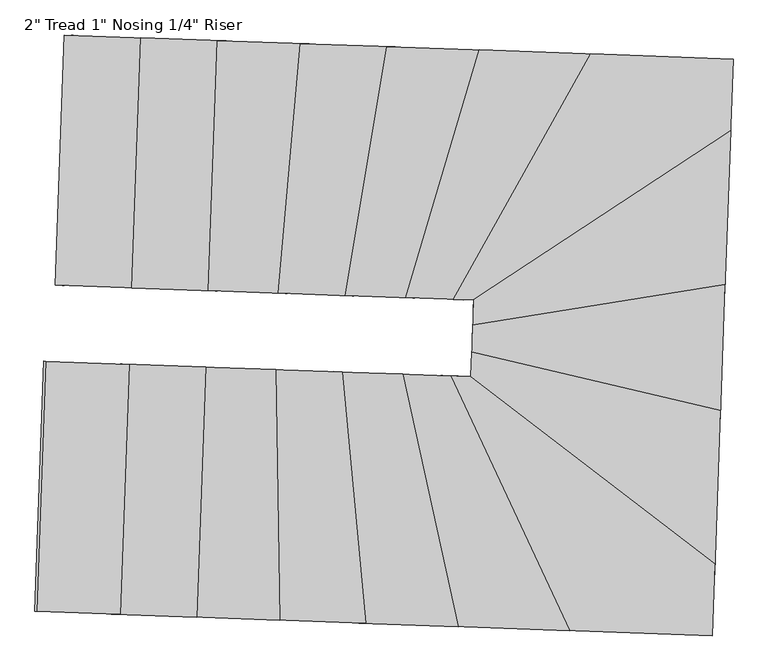
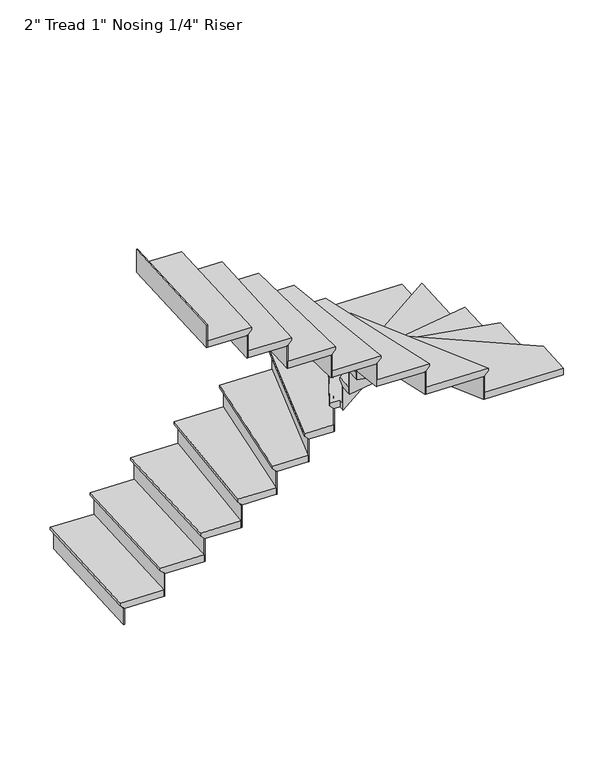
"""IFC4 building model written with IfcOpenShell, lengths in millimetres: stair flight geometry."""

from ifc_helpers import new_model, si_unit, origin, place, context, project, spatial, faceted_brep, source, transform, mapped, element, save


def stair_flight_9054a24f(model_context):
    return source(origin(), model_context, "Body", "Brep", [
        faceted_brep([(-10039.2744432, -1277.1215258, 150.2833333), (-10039.2744432, -1277.1215258, 169.3333333), (-10006.394185, -363.3128759, 169.3333333), (-10006.394185, -363.3128759, 150.2833333), (-10013.8908696, -1278.0348663, 124.8833333), (-9981.0106114, -364.2262164, 124.8833333), (-9734.6715599, -1288.0816118, 169.3333333), (-9701.7913017, -374.272962, 169.3333333), (-9981.0106114, -364.2262164, 118.5333333), (-9701.7913017, -374.272962, 118.5333333), (-9734.6715599, -1288.0816118, 118.5333333), (-10013.8908696, -1278.0348663, 118.5333333)], [[[0, 1, 2, 3]], [[4, 0, 3, 5]], [[2, 1, 6, 7]], [[8, 9, 10, 11]], [[2, 7, 9, 8, 5, 3]], [[8, 11, 4, 5]], [[6, 1, 0, 4, 11, 10]], [[7, 6, 10, 9]]]),
        faceted_brep([(-10013.8908696, -1278.0348663, 118.5333333), (-10013.8908696, -1278.0348663, 0.0), (-10007.5449762, -1278.2632014, 0.0), (-10007.5449762, -1278.2632014, 118.5333333), (-9981.0106114, -364.2262164, 118.5333333), (-9974.664718, -364.4545515, 118.5333333), (-9974.664718, -364.4545515, 0.0), (-9981.0106114, -364.2262164, 0.0)], [[[0, 1, 2, 3]], [[4, 5, 6, 7]], [[1, 0, 4, 7]], [[2, 1, 7, 6]], [[3, 2, 6, 5]], [[0, 3, 5, 4]]]),
        faceted_brep([(-9734.6715599, -1288.0816118, 287.8666667), (-9734.6715599, -1288.0816118, 118.5333333), (-9728.3256665, -1288.309947, 118.5333333), (-9728.3256665, -1288.309947, 287.8666667), (-9701.7913017, -374.272962, 287.8666667), (-9695.4454083, -374.5012971, 287.8666667), (-9695.4454083, -374.5012971, 118.5333333), (-9701.7913017, -374.272962, 118.5333333)], [[[0, 1, 2, 3]], [[4, 5, 6, 7]], [[1, 0, 4, 7]], [[2, 1, 7, 6]], [[3, 2, 6, 5]], [[0, 3, 5, 4]]]),
        faceted_brep([(-9727.1748753, -373.3596215, 338.6666667), (-9760.0551335, -1287.1682713, 338.6666667), (-9455.4522502, -1298.1283574, 338.6666667), (-9422.571992, -384.3197075, 338.6666667), (-9701.7913017, -374.272962, 287.8666667), (-9422.571992, -384.3197075, 287.8666667), (-9455.4522502, -1298.1283574, 287.8666667), (-9734.6715599, -1288.0816118, 287.8666667), (-9701.7913017, -374.272962, 294.2166667), (-9727.1748753, -373.3596215, 319.6166667), (-9734.6715599, -1288.0816118, 294.2166667), (-9760.0551335, -1287.1682713, 319.6166667)], [[[0, 1, 2, 3]], [[4, 5, 6, 7]], [[0, 3, 5, 4, 8, 9]], [[4, 7, 10, 8]], [[2, 1, 11, 10, 7, 6]], [[3, 2, 6, 5]], [[11, 1, 0, 9]], [[10, 11, 9, 8]]]),
        faceted_brep([(-9455.4522502, -1298.1283574, 457.2), (-9455.4522502, -1298.1283574, 287.8666667), (-9449.1063568, -1298.3566925, 287.8666667), (-9449.1063568, -1298.3566925, 457.2), (-9422.571992, -384.3197075, 457.2), (-9416.2260986, -384.5480426, 457.2), (-9416.2260986, -384.5480426, 287.8666667), (-9422.571992, -384.3197075, 287.8666667)], [[[0, 1, 2, 3]], [[4, 5, 6, 7]], [[1, 0, 4, 7]], [[2, 1, 7, 6]], [[3, 2, 6, 5]], [[0, 3, 5, 4]]]),
        faceted_brep([(-9447.9555656, -383.406367, 508.0), (-9480.8358238, -1297.2150169, 508.0), (-9199.9504308, -1307.3217107, 508.0), (-9119.566643, -395.2223118, 508.0), (-9422.571992, -384.3197075, 457.2), (-9119.566643, -395.2223118, 457.2), (-9199.9504308, -1307.3217107, 457.2), (-9455.4522502, -1298.1283574, 457.2), (-9422.571992, -384.3197075, 463.55), (-9447.9555656, -383.406367, 488.95), (-9455.4522502, -1298.1283574, 463.55), (-9480.8358238, -1297.2150169, 488.95)], [[[0, 1, 2, 3]], [[4, 5, 6, 7]], [[0, 3, 5, 4, 8, 9]], [[4, 7, 10, 8]], [[2, 1, 11, 10, 7, 6]], [[3, 2, 6, 5]], [[11, 1, 0, 9]], [[10, 11, 9, 8]]]),
        faceted_brep([(-9199.9504308, -1307.3217107, 626.5333333), (-9199.9504308, -1307.3217107, 457.2), (-9193.5959688, -1307.5503542, 457.2), (-9193.5959688, -1307.5503542, 626.5333333), (-9119.566643, -395.2223118, 626.5333333), (-9113.212181, -395.4509552, 626.5333333), (-9113.212181, -395.4509552, 457.2), (-9119.566643, -395.2223118, 457.2)], [[[0, 1, 2, 3]], [[4, 5, 6, 7]], [[1, 0, 4, 7]], [[2, 1, 7, 6]], [[3, 2, 6, 5]], [[0, 3, 5, 4]]]),
        faceted_brep([(-9144.9844911, -394.3077381, 677.3333333), (-9225.3682789, -1306.407137, 677.3333333), (-8955.9416356, -1316.1015272, 677.3333333), (-8804.7818676, -406.5487582, 677.3333333), (-9119.566643, -395.2223118, 626.5333333), (-8804.7818676, -406.5487582, 626.5333333), (-8955.9416356, -1316.1015272, 626.5333333), (-9199.9504308, -1307.3217107, 626.5333333), (-9119.566643, -395.2223118, 632.8833333), (-9144.9844911, -394.3077381, 658.2833333), (-9199.9504308, -1307.3217107, 632.8833333), (-9225.3682789, -1306.407137, 658.2833333)], [[[0, 1, 2, 3]], [[4, 5, 6, 7]], [[0, 3, 5, 4, 8, 9]], [[4, 7, 10, 8]], [[2, 1, 11, 10, 7, 6]], [[3, 2, 6, 5]], [[11, 1, 0, 9]], [[10, 11, 9, 8]]]),
        faceted_brep([(-8955.9416356, -1316.1015272, 795.8666667), (-8955.9416356, -1316.1015272, 626.5333333), (-8949.5428047, -1316.3317671, 626.5333333), (-8949.5428047, -1316.3317671, 795.8666667), (-8804.7818676, -406.5487582, 795.8666667), (-8798.3830367, -406.7789981, 795.8666667), (-8798.3830367, -406.7789981, 626.5333333), (-8804.7818676, -406.5487582, 626.5333333)], [[[0, 1, 2, 3]], [[4, 5, 6, 7]], [[1, 0, 4, 7]], [[2, 1, 7, 6]], [[3, 2, 6, 5]], [[0, 3, 5, 4]]]),
        faceted_brep([(-8830.3771913, -405.6277986, 846.6666667), (-8981.5369593, -1315.1805676, 846.6666667), (-8734.4577413, -1324.0708626, 846.6666667), (-8466.5990966, -418.7171009, 846.6666667), (-8804.7818676, -406.5487582, 795.8666667), (-8466.5990966, -418.7171009, 795.8666667), (-8734.4577413, -1324.0708626, 795.8666667), (-8955.9416356, -1316.1015272, 795.8666667), (-8804.7818676, -406.5487582, 802.2166667), (-8830.3771913, -405.6277986, 827.6166667), (-8955.9416356, -1316.1015272, 802.2166667), (-8981.5369593, -1315.1805676, 827.6166667)], [[[0, 1, 2, 3]], [[4, 5, 6, 7]], [[0, 3, 5, 4, 8, 9]], [[4, 7, 10, 8]], [[2, 1, 11, 10, 7, 6]], [[3, 2, 6, 5]], [[11, 1, 0, 9]], [[10, 11, 9, 8]]]),
        faceted_brep([(-8734.4577413, -1324.0708626, 965.2), (-8734.4577413, -1324.0708626, 795.8666667), (-8727.9054047, -1324.3066258, 795.8666667), (-8727.9054047, -1324.3066258, 965.2), (-8466.5990966, -418.7171009, 965.2), (-8460.0467599, -418.9528642, 965.2), (-8460.0467599, -418.9528642, 795.8666667), (-8466.5990966, -418.7171009, 795.8666667)], [[[0, 1, 2, 3]], [[4, 5, 6, 7]], [[1, 0, 4, 7]], [[2, 1, 7, 6]], [[3, 2, 6, 5]], [[0, 3, 5, 4]]]),
        faceted_brep([(-8492.8084432, -417.7740478, 1016.0), (-8760.667088, -1323.1278095, 1016.0), (-8558.2251501, -1330.4119856, 1016.0), (-8056.8234634, -433.4614663, 1016.0), (-8466.5990966, -418.7171009, 965.2), (-8056.8234634, -433.4614663, 965.2), (-8558.2251501, -1330.4119856, 965.2), (-8734.4577413, -1324.0708626, 965.2), (-8466.5990966, -418.7171009, 971.55), (-8492.8084432, -417.7740478, 996.95), (-8734.4577413, -1324.0708626, 971.55), (-8760.667088, -1323.1278095, 996.95)], [[[0, 1, 2, 3]], [[4, 5, 6, 7]], [[0, 3, 5, 4, 8, 9]], [[4, 7, 10, 8]], [[2, 1, 11, 10, 7, 6]], [[3, 2, 6, 5]], [[11, 1, 0, 9]], [[10, 11, 9, 8]]]),
        faceted_brep([(-8558.2251501, -1330.4119856, 1134.5333333), (-8558.2251501, -1330.4119856, 965.2), (-8551.0937819, -1330.6685834, 965.2), (-8551.0937819, -1330.6685834, 1134.5333333), (-8056.8234634, -433.4614663, 1134.5333333), (-8049.6920951, -433.718064, 1134.5333333), (-8049.6920951, -433.718064, 965.2), (-8056.8234634, -433.4614663, 965.2)], [[[0, 1, 2, 3]], [[4, 5, 6, 7]], [[1, 0, 4, 7]], [[2, 1, 7, 6]], [[3, 2, 6, 5]], [[0, 3, 5, 4]]]),
        faceted_brep([(-7576.4021107, -744.6189573, 1185.3333333), (-7565.8418401, -451.1277497, 1185.3333333), (-8085.3489363, -432.4350754, 1185.3333333), (-8586.750623, -1329.3855947, 1185.3333333), (-8512.5307482, -1332.0561414, 1185.3333333), (-8513.5934983, -1361.5921107, 1185.3333333), (-7565.8418401, -451.1277497, 1134.5333333), (-7576.4021107, -744.6189573, 1134.5333333), (-8513.5934983, -1361.5921107, 1134.5333333), (-8512.5307482, -1332.0561414, 1134.5333333), (-8558.2251501, -1330.4119856, 1134.5333333), (-8056.8234634, -433.4614663, 1134.5333333), (-8056.8234634, -433.4614663, 1140.8833333), (-8085.3489363, -432.4350754, 1166.2833333), (-8558.2251501, -1330.4119856, 1140.8833333), (-8586.750623, -1329.3855947, 1166.2833333)], [[[0, 1, 2, 3, 4, 5]], [[6, 7, 8, 9, 10, 11]], [[1, 0, 7, 6]], [[2, 1, 6, 11, 12, 13]], [[11, 10, 14, 12]], [[4, 3, 15, 14, 10, 9]], [[5, 4, 9, 8]], [[0, 5, 8, 7]], [[15, 3, 2, 13]], [[14, 15, 13, 12]]]),
        faceted_brep([(-8513.5934983, -1361.5921107, 1303.8666667), (-8513.5934983, -1361.5921107, 1134.5333333), (-8513.8736844, -1369.3790464, 1134.5333333), (-8513.8736844, -1369.3790464, 1303.8666667), (-7576.4021107, -744.6189573, 1303.8666667), (-7576.6822968, -752.405893, 1303.8666667), (-7576.6822968, -752.405893, 1134.5333333), (-7576.4021107, -744.6189573, 1134.5333333)], [[[0, 1, 2, 3]], [[4, 5, 6, 7]], [[1, 0, 4, 7]], [[2, 1, 7, 6]], [[3, 2, 6, 5]], [[0, 3, 5, 4]]]),
        faceted_brep([(-7575.2813665, -713.4712147, 1354.6666667), (-8512.472754, -1330.4443681, 1354.6666667), (-8516.7022393, -1447.9902872, 1354.6666667), (-7596.4124368, -1300.7462523, 1354.6666667), (-7576.4021107, -744.6189573, 1303.8666667), (-7596.4124368, -1300.7462523, 1303.8666667), (-8516.7022393, -1447.9902872, 1303.8666667), (-8513.5934983, -1361.5921107, 1303.8666667), (-7576.4021107, -744.6189573, 1310.2166667), (-7575.2813665, -713.4712147, 1335.6166667), (-8513.5934983, -1361.5921107, 1310.2166667), (-8512.472754, -1330.4443681, 1335.6166667)], [[[0, 1, 2, 3]], [[4, 5, 6, 7]], [[0, 3, 5, 4, 8, 9]], [[4, 7, 10, 8]], [[2, 1, 11, 10, 7, 6]], [[3, 2, 6, 5]], [[11, 1, 0, 9]], [[10, 11, 9, 8]]]),
        faceted_brep([(-8516.7022393, -1447.9902872, 1473.2), (-8516.7022393, -1447.9902872, 1303.8666667), (-8516.934968, -1454.458287, 1303.8666667), (-8516.934968, -1454.458287, 1473.2), (-7596.4124368, -1300.7462523, 1473.2), (-7596.6451655, -1307.2142521, 1473.2), (-7596.6451655, -1307.2142521, 1303.8666667), (-7596.4124368, -1300.7462523, 1303.8666667)], [[[0, 1, 2, 3]], [[4, 5, 6, 7]], [[1, 0, 4, 7]], [[2, 1, 7, 6]], [[3, 2, 6, 5]], [[0, 3, 5, 4]]]),
        faceted_brep([(-7595.481522, -1274.874253, 1524.0), (-8515.7713244, -1422.1182879, 1524.0), (-8520.2678323, -1547.0853038, 1524.0), (-7612.9403349, -1760.0898551, 1524.0), (-7596.4124368, -1300.7462523, 1473.2), (-7612.9403349, -1760.0898551, 1473.2), (-8520.2678323, -1547.0853038, 1473.2), (-8516.7022393, -1447.9902872, 1473.2), (-7596.4124368, -1300.7462523, 1479.55), (-7595.481522, -1274.874253, 1504.95), (-8516.7022393, -1447.9902872, 1479.55), (-8515.7713244, -1422.1182879, 1504.95)], [[[0, 1, 2, 3]], [[4, 5, 6, 7]], [[0, 3, 5, 4, 8, 9]], [[4, 7, 10, 8]], [[2, 1, 11, 10, 7, 6]], [[3, 2, 6, 5]], [[11, 1, 0, 9]], [[10, 11, 9, 8]]]),
        faceted_brep([(-8520.2678323, -1547.0853038, 1642.5333333), (-8520.2678323, -1547.0853038, 1473.2), (-8520.500561, -1553.5533036, 1473.2), (-8520.500561, -1553.5533036, 1642.5333333), (-7612.9403349, -1760.0898551, 1642.5333333), (-7613.1730636, -1766.5578549, 1642.5333333), (-7613.1730636, -1766.5578549, 1473.2), (-7612.9403349, -1760.0898551, 1473.2)], [[[0, 1, 2, 3]], [[4, 5, 6, 7]], [[1, 0, 4, 7]], [[2, 1, 7, 6]], [[3, 2, 6, 5]], [[0, 3, 5, 4]]]),
        faceted_brep([(-7612.0094201, -1734.2178558, 1693.3333333), (-8519.3369174, -1521.2133045, 1693.3333333), (-8522.5774937, -1611.2754511, 1693.3333333), (-8568.6431579, -1609.6179367, 1693.3333333), (-7633.3303199, -2326.7686368, 1693.3333333), (-7612.9403349, -1760.0898551, 1642.5333333), (-7633.3303199, -2326.7686368, 1642.5333333), (-8568.6431579, -1609.6179367, 1642.5333333), (-8522.5774937, -1611.2754511, 1642.5333333), (-8520.2678323, -1547.0853038, 1642.5333333), (-7612.9403349, -1760.0898551, 1648.8833333), (-7612.0094201, -1734.2178558, 1674.2833333), (-8520.2678323, -1547.0853038, 1648.8833333), (-8519.3369174, -1521.2133045, 1674.2833333)], [[[0, 1, 2, 3, 4]], [[5, 6, 7, 8, 9]], [[0, 4, 6, 5, 10, 11]], [[5, 9, 12, 10]], [[2, 1, 13, 12, 9, 8]], [[3, 2, 8, 7]], [[4, 3, 7, 6]], [[13, 1, 0, 11]], [[12, 13, 11, 10]]]),
        faceted_brep([(-8568.6431579, -1609.6179367, 1811.8666667), (-8568.6431579, -1609.6179367, 1642.5333333), (-8579.5929645, -1609.2239456, 1642.5333333), (-8579.5929645, -1609.2239456, 1811.8666667), (-7633.3303199, -2326.7686368, 1811.8666667), (-7633.610506, -2334.5555724, 1811.8666667), (-7633.610506, -2334.5555724, 1642.5333333), (-7633.3303199, -2326.7686368, 1642.5333333)], [[[0, 1, 2, 3]], [[4, 5, 6, 7]], [[1, 0, 4, 7]], [[2, 1, 7, 6]], [[3, 2, 6, 5]], [[0, 3, 5, 4]]]),
        faceted_brep([(-8189.6816712, -2538.2452939, 1862.6666667), (-7641.649102, -2557.9643591, 1862.6666667), (-7632.2095756, -2295.6208941, 1862.6666667), (-8524.8439316, -1611.1939011, 1862.6666667), (-8625.3228415, -1607.5785134, 1862.6666667), (-7641.649102, -2557.9643591, 1811.8666667), (-8189.6816712, -2538.2452939, 1811.8666667), (-8625.3228415, -1607.5785134, 1811.8666667), (-8568.6431579, -1609.6179367, 1811.8666667), (-7633.3303199, -2326.7686368, 1811.8666667), (-7633.3303199, -2326.7686368, 1818.2166667), (-7632.2095756, -2295.6208941, 1843.6166667), (-8568.6431579, -1609.6179367, 1818.2166667), (-8524.8439316, -1611.1939011, 1843.6166667)], [[[0, 1, 2, 3, 4]], [[5, 6, 7, 8, 9]], [[1, 0, 6, 5]], [[2, 1, 5, 9, 10, 11]], [[9, 8, 12, 10]], [[4, 3, 13, 12, 8, 7]], [[0, 4, 7, 6]], [[13, 3, 2, 11]], [[12, 13, 11, 10]]]),
        faceted_brep([(-8625.3228415, -1607.5785134, 1981.2), (-8625.3228415, -1607.5785134, 1811.8666667), (-8632.4542098, -1607.3219157, 1811.8666667), (-8632.4542098, -1607.3219157, 1981.2), (-8189.6816712, -2538.2452939, 1981.2), (-8196.8130394, -2537.9886962, 1981.2), (-8196.8130394, -2537.9886962, 1811.8666667), (-8189.6816712, -2538.2452939, 1811.8666667)], [[[0, 1, 2, 3]], [[4, 5, 6, 7]], [[1, 0, 4, 7]], [[2, 1, 7, 6]], [[3, 2, 6, 5]], [[0, 3, 5, 4]]]),
        faceted_brep([(-8161.1561983, -2539.2716849, 2032.0), (-8596.7973686, -1608.6049044, 2032.0), (-8796.9231803, -1601.404066, 2032.0), (-8594.8250519, -2523.6676042, 2032.0), (-8189.6816712, -2538.2452939, 1981.2), (-8594.8250519, -2523.6676042, 1981.2), (-8796.9231803, -1601.404066, 1981.2), (-8625.3228415, -1607.5785134, 1981.2), (-8189.6816712, -2538.2452939, 1987.55), (-8161.1561983, -2539.2716849, 2012.95), (-8625.3228415, -1607.5785134, 1987.55), (-8596.7973686, -1608.6049044, 2012.95)], [[[0, 1, 2, 3]], [[4, 5, 6, 7]], [[0, 3, 5, 4, 8, 9]], [[4, 7, 10, 8]], [[2, 1, 11, 10, 7, 6]], [[3, 2, 6, 5]], [[11, 1, 0, 9]], [[10, 11, 9, 8]]]),
        faceted_brep([(-8796.9231803, -1601.404066, 2150.5333333), (-8796.9231803, -1601.404066, 1981.2), (-8803.475517, -1601.1683028, 1981.2), (-8803.475517, -1601.1683028, 2150.5333333), (-8594.8250519, -2523.6676042, 2150.5333333), (-8601.3773886, -2523.4318409, 2150.5333333), (-8601.3773886, -2523.4318409, 1981.2), (-8594.8250519, -2523.6676042, 1981.2)], [[[0, 1, 2, 3]], [[4, 5, 6, 7]], [[1, 0, 4, 7]], [[2, 1, 7, 6]], [[3, 2, 6, 5]], [[0, 3, 5, 4]]]),
        faceted_brep([(-8568.6157052, -2524.6106573, 2201.3333333), (-8770.7138336, -1602.3471191, 2201.3333333), (-9017.1790286, -1593.4789176, 2201.3333333), (-8931.779777, -2511.5434485, 2201.3333333), (-8594.8250519, -2523.6676042, 2150.5333333), (-8931.779777, -2511.5434485, 2150.5333333), (-9017.1790286, -1593.4789176, 2150.5333333), (-8796.9231803, -1601.404066, 2150.5333333), (-8594.8250519, -2523.6676042, 2156.8833333), (-8568.6157052, -2524.6106573, 2182.2833333), (-8796.9231803, -1601.404066, 2156.8833333), (-8770.7138336, -1602.3471191, 2182.2833333)], [[[0, 1, 2, 3]], [[4, 5, 6, 7]], [[0, 3, 5, 4, 8, 9]], [[4, 7, 10, 8]], [[2, 1, 11, 10, 7, 6]], [[3, 2, 6, 5]], [[11, 1, 0, 9]], [[10, 11, 9, 8]]]),
        faceted_brep([(-9017.1790286, -1593.4789176, 2319.8666667), (-9017.1790286, -1593.4789176, 2150.5333333), (-9023.5778595, -1593.2486777, 2150.5333333), (-9023.5778595, -1593.2486777, 2319.8666667), (-8931.779777, -2511.5434485, 2319.8666667), (-8938.1786079, -2511.3132086, 2319.8666667), (-8938.1786079, -2511.3132086, 2150.5333333), (-8931.779777, -2511.5434485, 2150.5333333)], [[[0, 1, 2, 3]], [[4, 5, 6, 7]], [[1, 0, 4, 7]], [[2, 1, 7, 6]], [[3, 2, 6, 5]], [[0, 3, 5, 4]]]),
        faceted_brep([(-8906.1844533, -2512.4644081, 2370.6666667), (-8991.5837049, -1594.3998772, 2370.6666667), (-9260.8328726, -1584.7118729, 2370.6666667), (-9246.2096012, -2500.2297738, 2370.6666667), (-8931.779777, -2511.5434485, 2319.8666667), (-9246.2096012, -2500.2297738, 2319.8666667), (-9260.8328726, -1584.7118729, 2319.8666667), (-9017.1790286, -1593.4789176, 2319.8666667), (-8931.779777, -2511.5434485, 2326.2166667), (-8906.1844533, -2512.4644081, 2351.6166667), (-9017.1790286, -1593.4789176, 2326.2166667), (-8991.5837049, -1594.3998772, 2351.6166667)], [[[0, 1, 2, 3]], [[4, 5, 6, 7]], [[0, 3, 5, 4, 8, 9]], [[4, 7, 10, 8]], [[2, 1, 11, 10, 7, 6]], [[3, 2, 6, 5]], [[11, 1, 0, 9]], [[10, 11, 9, 8]]]),
        faceted_brep([(-9260.8328726, -1584.7118729, 2489.2), (-9260.8328726, -1584.7118729, 2319.8666667), (-9267.1873346, -1584.4832295, 2319.8666667), (-9267.1873346, -1584.4832295, 2489.2), (-9246.2096012, -2500.2297738, 2489.2), (-9252.5640632, -2500.0011303, 2489.2), (-9252.5640632, -2500.0011303, 2319.8666667), (-9246.2096012, -2500.2297738, 2319.8666667)], [[[0, 1, 2, 3]], [[4, 5, 6, 7]], [[1, 0, 4, 7]], [[2, 1, 7, 6]], [[3, 2, 6, 5]], [[0, 3, 5, 4]]]),
        faceted_brep([(-9220.7917531, -2501.1443475, 2540.0), (-9235.4150245, -1585.6264467, 2540.0), (-9516.266143, -1575.5209861, 2540.0), (-9549.1464012, -2489.329636, 2540.0), (-9246.2096012, -2500.2297738, 2489.2), (-9549.1464012, -2489.329636, 2489.2), (-9516.266143, -1575.5209861, 2489.2), (-9260.8328726, -1584.7118729, 2489.2), (-9246.2096012, -2500.2297738, 2495.55), (-9220.7917531, -2501.1443475, 2520.95), (-9260.8328726, -1584.7118729, 2495.55), (-9235.4150245, -1585.6264467, 2520.95)], [[[0, 1, 2, 3]], [[4, 5, 6, 7]], [[0, 3, 5, 4, 8, 9]], [[4, 7, 10, 8]], [[2, 1, 11, 10, 7, 6]], [[3, 2, 6, 5]], [[11, 1, 0, 9]], [[10, 11, 9, 8]]]),
        faceted_brep([(-9516.266143, -1575.5209861, 2658.5333333), (-9516.266143, -1575.5209861, 2489.2), (-9522.6120364, -1575.292651, 2489.2), (-9522.6120364, -1575.292651, 2658.5333333), (-9549.1464012, -2489.329636, 2658.5333333), (-9555.4922946, -2489.1013009, 2658.5333333), (-9555.4922946, -2489.1013009, 2489.2), (-9549.1464012, -2489.329636, 2489.2)], [[[0, 1, 2, 3]], [[4, 5, 6, 7]], [[1, 0, 4, 7]], [[2, 1, 7, 6]], [[3, 2, 6, 5]], [[0, 3, 5, 4]]]),
        faceted_brep([(-9523.7628276, -2490.2429765, 2709.3333333), (-9490.8825694, -1576.4343266, 2709.3333333), (-9795.4854527, -1565.4742405, 2709.3333333), (-9828.3657109, -2479.2828904, 2709.3333333), (-9549.1464012, -2489.329636, 2658.5333333), (-9828.3657109, -2479.2828904, 2658.5333333), (-9795.4854527, -1565.4742405, 2658.5333333), (-9516.266143, -1575.5209861, 2658.5333333), (-9549.1464012, -2489.329636, 2664.8833333), (-9523.7628276, -2490.2429765, 2690.2833333), (-9516.266143, -1575.5209861, 2664.8833333), (-9490.8825694, -1576.4343266, 2690.2833333)], [[[0, 1, 2, 3]], [[4, 5, 6, 7]], [[0, 3, 5, 4, 8, 9]], [[4, 7, 10, 8]], [[2, 1, 11, 10, 7, 6]], [[3, 2, 6, 5]], [[11, 1, 0, 9]], [[10, 11, 9, 8]]]),
        faceted_brep([(-9795.4854527, -1565.4742405, 2827.8666667), (-9795.4854527, -1565.4742405, 2658.5333333), (-9801.8313461, -1565.2459054, 2658.5333333), (-9801.8313461, -1565.2459054, 2827.8666667), (-9828.3657109, -2479.2828904, 2827.8666667), (-9834.7116043, -2479.0545553, 2827.8666667), (-9834.7116043, -2479.0545553, 2658.5333333), (-9828.3657109, -2479.2828904, 2658.5333333)], [[[0, 1, 2, 3]], [[4, 5, 6, 7]], [[1, 0, 4, 7]], [[2, 1, 7, 6]], [[3, 2, 6, 5]], [[0, 3, 5, 4]]]),
        faceted_brep([(-10074.7047624, -1555.427495, 2997.2), (-10074.7047624, -1555.427495, 2827.8666667), (-10081.0506558, -1555.1991598, 2827.8666667), (-10081.0506558, -1555.1991598, 2997.2), (-10107.5850206, -2469.2361449, 2997.2), (-10113.930914, -2469.0078097, 2997.2), (-10113.930914, -2469.0078097, 2827.8666667), (-10107.5850206, -2469.2361449, 2827.8666667)], [[[0, 1, 2, 3]], [[4, 5, 6, 7]], [[1, 0, 4, 7]], [[2, 1, 7, 6]], [[3, 2, 6, 5]], [[0, 3, 5, 4]]]),
        faceted_brep([(-9802.9821373, -2480.1962309, 2878.6666667), (-9770.1018791, -1566.387581, 2878.6666667), (-10074.7047624, -1555.427495, 2878.6666667), (-10107.5850206, -2469.2361449, 2878.6666667), (-9828.3657109, -2479.2828904, 2827.8666667), (-10107.5850206, -2469.2361449, 2827.8666667), (-10074.7047624, -1555.427495, 2827.8666667), (-9795.4854527, -1565.4742405, 2827.8666667), (-9828.3657109, -2479.2828904, 2834.2166667), (-9802.9821373, -2480.1962309, 2859.6166667), (-9795.4854527, -1565.4742405, 2834.2166667), (-9770.1018791, -1566.387581, 2859.6166667)], [[[0, 1, 2, 3]], [[4, 5, 6, 7]], [[0, 3, 5, 4, 8, 9]], [[4, 7, 10, 8]], [[2, 1, 11, 10, 7, 6]], [[3, 2, 6, 5]], [[11, 1, 0, 9]], [[10, 11, 9, 8]]]),
    ])


if __name__ == "__main__":
    model = new_model("IFC4")
    model_context = context("Model", 3, world=origin())
    ifc_project = project(units=[si_unit("LENGTHUNIT", "METRE", prefix="MILLI")], contexts=[model_context])
    site = spatial("IfcSite", under=ifc_project)
    building = spatial("IfcBuilding", under=site)
    placement = place(None, origin())
    stair_flight_shape = stair_flight_9054a24f(model_context)
    element("IfcStairFlight", 1, ObjectType="2\" Tread 1\" Nosing 1/4\" Riser", at=placement, inside=building, context=model_context, shape_type="MappedRepresentation", body=[
        mapped(stair_flight_shape, transform((0.0, 0.0, 0.0), x_axis=(1.0, 0.0, 0.0), y_axis=(0.0, 1.0, 0.0), z_axis=(0.0, 0.0, 1.0))),
    ])
    save(model, "model.ifc")
